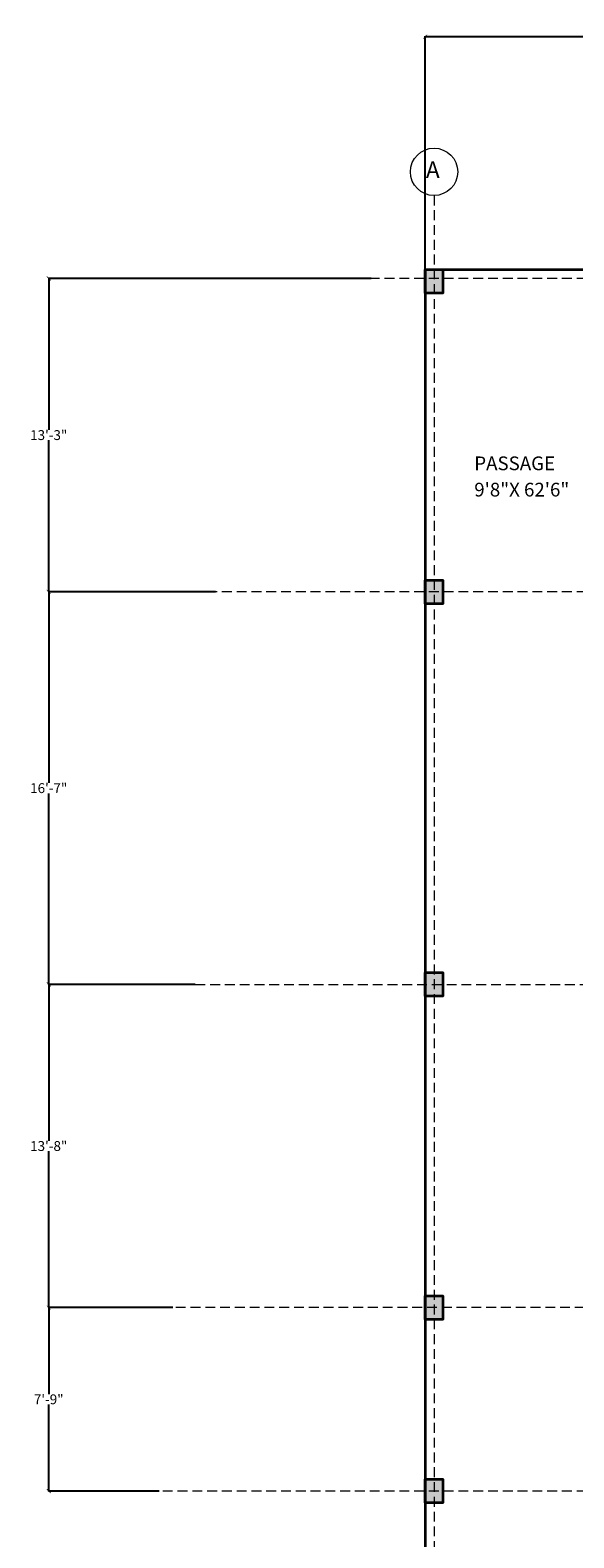
# Model space of a CAD drawing. Units: inches. Extents: x 782 to 2660, y -1008 to 166.
# Tile 2 of 12: x 782 to 1058, y -598 to 166. Entities that reach past the tile are written whole.
import ezdxf

# ---------------------------------------------------------------- set-up
doc = ezdxf.new("R2010")
doc.units = ezdxf.units.IN
doc.header["$MEASUREMENT"] = 0
doc.linetypes.add('DASHED', pattern=[0.75, 0.5, -0.25])
for name, color, linetype, lineweight in [('A-ANNO-DIMS', 4, 'Continuous', 18), ('A-AREA-IDEN', 4, 'Continuous', 18), ('A-COLS', 7, 'Continuous', 35), ('A-GRID', 8, 'DASHED', 13), ('A-GRID-IDEN', 7, 'Continuous', 18), ('A-WALL', 7, 'Continuous', 35)]:
    doc.layers.add(name, color=color, linetype=linetype, lineweight=lineweight)
doc.styles.get("Standard").update_dxf_attribs({"font": 'arial.ttf'})
doc.dimstyles.get("Standard").update_dxf_attribs({"dimtxt": 5, "dimasz": 2, "dimexe": 0.18, "dimexo": 0.0625, "dimgap": 0.09, "dimtad": 0, "dimtih": 1, "dimtoh": 1, "dimdec": 0, "dimzin": 0, "dimdsep": 46, "dimlunit": 3, "dimtxsty": 'Standard', "dimblk": 'ARCHTICK', "dimcen": 0.09, "dimadec": 0, "dimazin": 0, "dimtfac": 1, "dimtdec": 0, "dimtofl": 0, "dimtmove": 0, "dimatfit": 3, "dimfxl": 1, "dimtolj": 1, "dimtzin": 0, "dimarcsym": 0})

# ---------------------------------------------------------------- blocks, each defined once
blk = doc.blocks.new('COL-9X12')
h = blk.add_hatch(color=256)
h.dxf.hatch_style = 1
h.paths.add_polyline_path([(9, 12), (0, 12), (0, 0), (9, 0)])
blk.add_lwpolyline([(0, 12), (9, 12), (9, 0), (0, 0)], close=True)
blk = doc.blocks.new('_ArchTick')
at = {"color": 0, "linetype": 'ByBlock', "const_width": 0.15}
blk.add_lwpolyline([(-0.5, -0.5), (0.5, 0.5)], dxfattribs=at)
blk = doc.blocks.new('*D52')
at = {"layer": 'A-ANNO-DIMS', "color": 0, "lineweight": -2, "transparency": 16777216}
for p, q in [((982.68, 45.07), (982.68, 163.27)), ((982.68, 163.09), (1186.01, 163.09)), ((1406.68, 163.09), (1203.36, 163.09)), ((1406.68, 45.07), (1406.68, 163.27))]:
    blk.add_line(p, q, dxfattribs=at)
at = {"layer": 'Defpoints', "color": 0, "transparency": 16777216}
for p in [(1406.68, 163.09), (982.68, 45.01), (1406.68, 45.01)]:
    blk.add_point(p, dxfattribs=at)
at = {"layer": 'A-ANNO-DIMS', "color": 0, "lineweight": -2, "transparency": 16777216, "xscale": 2, "yscale": 2, "zscale": 2, "rotation": 180}
blk.add_blockref('_ArchTick', (982.68, 163.09), dxfattribs=at)
at = {"layer": 'A-ANNO-DIMS', "color": 0, "lineweight": -2, "transparency": 16777216, "xscale": 2, "yscale": 2, "zscale": 2}
blk.add_blockref('_ArchTick', (1406.68, 163.09), dxfattribs=at)
at = {"layer": 'A-ANNO-DIMS', "color": 0, "transparency": 16777216, "insert": (1194.68, 163.09), "char_height": 5, "attachment_point": 5}
blk.add_mtext('\\A1;35\'-4"', dxfattribs=at)
blk = doc.blocks.new('*D58')
at = {"layer": 'A-ANNO-DIMS', "color": 0, "lineweight": -2, "transparency": 16777216}
for p, q in [((955.19, 40.51), (791.5, 40.51)), ((791.68, 40.51), (791.68, -36.35)), ((791.68, -118.49), (791.68, -41.64)), ((876.26, -118.49), (791.5, -118.49))]:
    blk.add_line(p, q, dxfattribs=at)
at = {"layer": 'Defpoints', "color": 0, "transparency": 16777216}
for p in [(791.68, 40.51), (955.26, 40.51), (876.32, -118.49)]:
    blk.add_point(p, dxfattribs=at)
at = {"layer": 'A-ANNO-DIMS', "color": 0, "lineweight": -2, "transparency": 16777216, "xscale": 2, "yscale": 2, "zscale": 2}
for p, rotation in [((791.68, 40.51), 90), ((791.68, -118.49), 270)]:
    blk.add_blockref('_ArchTick', p, dxfattribs=dict(at, rotation=rotation))
at = {"layer": 'A-ANNO-DIMS', "color": 0, "transparency": 16777216, "insert": (791.68, -38.99), "char_height": 5, "attachment_point": 5}
blk.add_mtext('\\A1;13\'-3"', dxfattribs=at)
blk = doc.blocks.new('*D59')
at = {"layer": 'A-ANNO-DIMS', "color": 0, "lineweight": -2, "transparency": 16777216}
for p, q in [((876.26, -118.49), (791.5, -118.49)), ((791.68, -118.49), (791.68, -215.38)), ((791.68, -317.56), (791.68, -220.67)), ((866.02, -317.56), (791.5, -317.56))]:
    blk.add_line(p, q, dxfattribs=at)
at = {"layer": 'Defpoints', "color": 0, "transparency": 16777216}
for p in [(791.68, -118.49), (876.32, -118.49), (866.08, -317.56)]:
    blk.add_point(p, dxfattribs=at)
at = {"layer": 'A-ANNO-DIMS', "color": 0, "lineweight": -2, "transparency": 16777216, "xscale": 2, "yscale": 2, "zscale": 2}
for p, rotation in [((791.68, -118.49), 90), ((791.68, -317.56), 270)]:
    blk.add_blockref('_ArchTick', p, dxfattribs=dict(at, rotation=rotation))
at = {"layer": 'A-ANNO-DIMS', "color": 0, "transparency": 16777216, "insert": (791.68, -218.03), "char_height": 5, "attachment_point": 5}
blk.add_mtext('\\A1;16\'-7"', dxfattribs=at)
blk = doc.blocks.new('*D60')
at = {"layer": 'A-ANNO-DIMS', "color": 0, "lineweight": -2, "transparency": 16777216}
for p, q in [((866.02, -317.56), (791.5, -317.56)), ((791.68, -317.56), (791.68, -396.88)), ((791.68, -481.49), (791.68, -402.17)), ((854.67, -481.49), (791.5, -481.49))]:
    blk.add_line(p, q, dxfattribs=at)
at = {"layer": 'Defpoints', "color": 0, "transparency": 16777216}
for p in [(791.68, -317.56), (866.08, -317.56), (854.73, -481.49)]:
    blk.add_point(p, dxfattribs=at)
at = {"layer": 'A-ANNO-DIMS', "color": 0, "lineweight": -2, "transparency": 16777216, "xscale": 2, "yscale": 2, "zscale": 2}
for p, rotation in [((791.68, -317.56), 90), ((791.68, -481.49), 270)]:
    blk.add_blockref('_ArchTick', p, dxfattribs=dict(at, rotation=rotation))
at = {"layer": 'A-ANNO-DIMS', "color": 0, "transparency": 16777216, "insert": (791.68, -399.53), "char_height": 5, "attachment_point": 5}
blk.add_mtext('\\A1;13\'-8"', dxfattribs=at)
blk = doc.blocks.new('*D61')
at = {"layer": 'A-ANNO-DIMS', "color": 0, "lineweight": -2, "transparency": 16777216}
for p, q in [((854.67, -481.49), (791.5, -481.49)), ((791.68, -481.49), (791.68, -525.35)), ((791.68, -574.49), (791.68, -530.64)), ((847.76, -574.49), (791.5, -574.49))]:
    blk.add_line(p, q, dxfattribs=at)
at = {"layer": 'Defpoints', "color": 0, "transparency": 16777216}
for p in [(791.68, -481.49), (854.73, -481.49), (847.83, -574.49)]:
    blk.add_point(p, dxfattribs=at)
at = {"layer": 'A-ANNO-DIMS', "color": 0, "lineweight": -2, "transparency": 16777216, "xscale": 2, "yscale": 2, "zscale": 2}
for p, rotation in [((791.68, -481.49), 90), ((791.68, -574.49), 270)]:
    blk.add_blockref('_ArchTick', p, dxfattribs=dict(at, rotation=rotation))
at = {"layer": 'A-ANNO-DIMS', "color": 0, "transparency": 16777216, "insert": (791.68, -527.99), "char_height": 5, "attachment_point": 5}
blk.add_mtext('\\A1;7\'-9"', dxfattribs=at)

msp = doc.modelspace()

# ---------------------------------------------------------------- linework, layer by layer
at = {"layer": 'A-GRID', "ltscale": 10}
for p, q in [((987.18, 82.53), (987.18, -949.03)), ((1499.56, 40.51), (955.26, 40.51)), ((1499.56, -118.49), (876.32, -118.49)), ((866.08, -317.56), (1499.56, -317.56)), ((1498.64, -481.49), (854.73, -481.49)), ((1499.56, -574.49), (847.83, -574.49))]:
    msp.add_line(p, q, dxfattribs=at)
at = {"layer": 'A-GRID-IDEN'}
msp.add_circle((987.18, 94.53), 12, dxfattribs=at)
at = {"layer": 'A-WALL'}
for q in [(982.68, -704.99), (1406.68, 45.01)]:
    msp.add_line((982.68, 45.01), q, dxfattribs=at)

# ---------------------------------------------------------------- block references
at = {"layer": 'A-COLS'}
for p in [(982.68, 33.01), (982.68, -124.49), (982.68, -323.56), (982.68, -487.49), (982.68, -580.49)]:
    msp.add_blockref('COL-9X12', p, dxfattribs=at)

# ---------------------------------------------------------------- texts
at = {"layer": 'A-AREA-IDEN'}
for s, height, p in [('PASSAGE', 6.958, (1007.58, -56.79)), ('9\'8"X 62\'6"', 6.9576, (1007.58, -70.13))]:
    msp.add_text(s, height=height, dxfattribs=at).set_placement(p)
at = {"layer": 'A-GRID-IDEN'}
msp.add_text('A', height=8.41, dxfattribs=at).set_placement((983.05, 91.42))

# ---------------------------------------------------------------- dimensions: what is measured, and where the dimension line sits
at = {"layer": 'A-ANNO-DIMS'}
dim = msp.add_linear_dim(base=(1406.68, 163.09), p1=(982.68, 45.01), p2=(1406.68, 45.01), dimstyle='Standard', override={"dimdec": 1, "dimlfac": 1, "dimrnd": 0, "dimzin": 1, "dimdsep": 46, "dimlunit": 4, "dimfrac": 2}, dxfattribs=at)
dim.commit()
dim.dimension.update_dxf_attribs({"geometry": '*D52', "text_midpoint": (1194.68, 163.09)})
for base, p1, p2, picture, middle in [((791.68, 40.51), (876.32, -118.49), (955.26, 40.51), '*D58', (791.68, -38.99)), ((791.68, -118.49), (866.08, -317.56), (876.32, -118.49), '*D59', (791.68, -218.03)), ((791.68, -317.56), (854.73, -481.49), (866.08, -317.56), '*D60', (791.68, -399.53)), ((791.68, -481.49), (847.83, -574.49), (854.73, -481.49), '*D61', (791.68, -527.99))]:
    dim = msp.add_linear_dim(base=base, p1=p1, p2=p2, angle=90, dimstyle='Standard', override={"dimdec": 1, "dimlfac": 1, "dimrnd": 0, "dimzin": 1, "dimdsep": 46, "dimlunit": 4, "dimfrac": 2}, dxfattribs=at)
    dim.commit()
    dim.dimension.update_dxf_attribs({"geometry": picture, "text_midpoint": middle})

doc.saveas('drawing.dxf')
